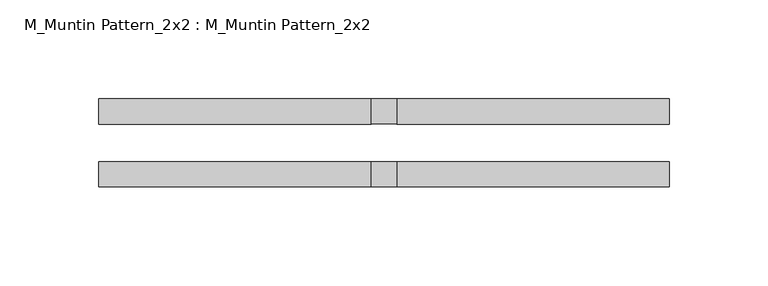
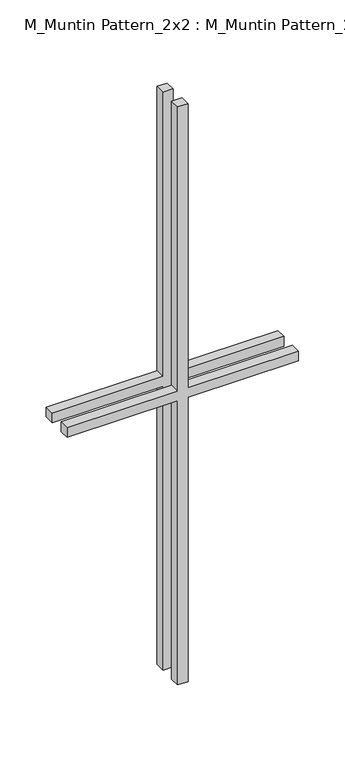
"""IFC4 building model written with IfcOpenShell, lengths in millimetres: proxy geometry, M_Muntin Pattern_2x2 : M_Muntin Pattern_2x2."""

from ifc_helpers import new_model, si_unit, frame, origin, place, context, project, spatial, polyline, outline, extrude, source, transform, mapped, element, save


def m_muntin_pattern_2x2_m_muntin_pattern_2x2_4fd78f17(model_context):
    return source(origin(), model_context, "Body", "SweptSolid", [
        extrude(outline(polyline([(386.5, -6.35), (386.5, -144.2375), (373.8, -144.2375), (373.8, -6.35), (0.0, -6.35), (0.0, 6.35), (373.8, 6.35), (373.8, 144.2375), (386.5, 144.2375), (386.5, 6.35), (760.3, 6.35), (760.3, -6.35), (386.5, -6.35)])), frame((0.0, -22.225, 0.0), z_axis=(0.0, 1.0, 0.0), x_axis=(0.0, 0.0, 1.0)), (0.0, 0.0, 1.0), 12.7),
        extrude(outline(polyline([(386.5, -6.35), (386.5, -144.2375), (373.8, -144.2375), (373.8, -6.35), (0.0, -6.35), (0.0, 6.35), (373.8, 6.35), (373.8, 144.2375), (386.5, 144.2375), (386.5, 6.35), (760.3, 6.35), (760.3, -6.35), (386.5, -6.35)])), frame((0.0, 9.525, 0.0), z_axis=(0.0, 1.0, 0.0), x_axis=(0.0, 0.0, 1.0)), (0.0, 0.0, 1.0), 12.7),
    ])


if __name__ == "__main__":
    model = new_model("IFC4")
    model_context = context("Model", 3, world=origin())
    ifc_project = project(units=[si_unit("LENGTHUNIT", "METRE", prefix="MILLI")], contexts=[model_context])
    site = spatial("IfcSite", under=ifc_project)
    building = spatial("IfcBuilding", under=site)
    placement = place(None, origin())
    m_muntin_pattern_2x2_m_muntin_pattern_2x2_shape = m_muntin_pattern_2x2_m_muntin_pattern_2x2_4fd78f17(model_context)
    element("IfcBuildingElementProxy", 1, Name="M_Muntin Pattern_2x2 : M_Muntin Pattern_2x2", ObjectType="M_Muntin Pattern_2x2 : M_Muntin Pattern_2x2", at=placement, inside=building, context=model_context, shape_type="MappedRepresentation", body=[
        mapped(m_muntin_pattern_2x2_m_muntin_pattern_2x2_shape, transform((0.0, 0.0, 0.0), x_axis=(1.0, 0.0, 0.0), y_axis=(0.0, 1.0, 0.0), z_axis=(0.0, 0.0, 1.0))),
    ])
    save(model, "model.ifc")

# Revit data of these elements
# Type "M_Muntin Pattern_2x2 : M_Muntin Pattern_2x2"
#   Width [instance default] = 3.937008 ft
#   Thickness = 0.041667 ft
#   Height [instance default] = 3.937008 ft
#   Distance = 0.0625 ft
#   Interior Material [instance default] = none
#   Exterior Material [instance default] = none
#   Default Elevation = 0
# Element 1 (IfcBuildingElementProxy, "M_Muntin Pattern_2x2 : M_Muntin Pattern_2x2")
#   Width = 0.94644 ft
#   Height = 2.494423 ft
#   Interior Material = Wood - Stained
#   Exterior Material = Clad - White
#   Materials on its faces: "Clad - White", "Wood - Stained"
# Materials
#   "Clad - White": class "Wood", colour RGB 242 242 238, transparency 0, Cost = 0
#   "Wood - Stained": class "Wood", colour RGB 224 178 126, transparency 0, Cost = 0
